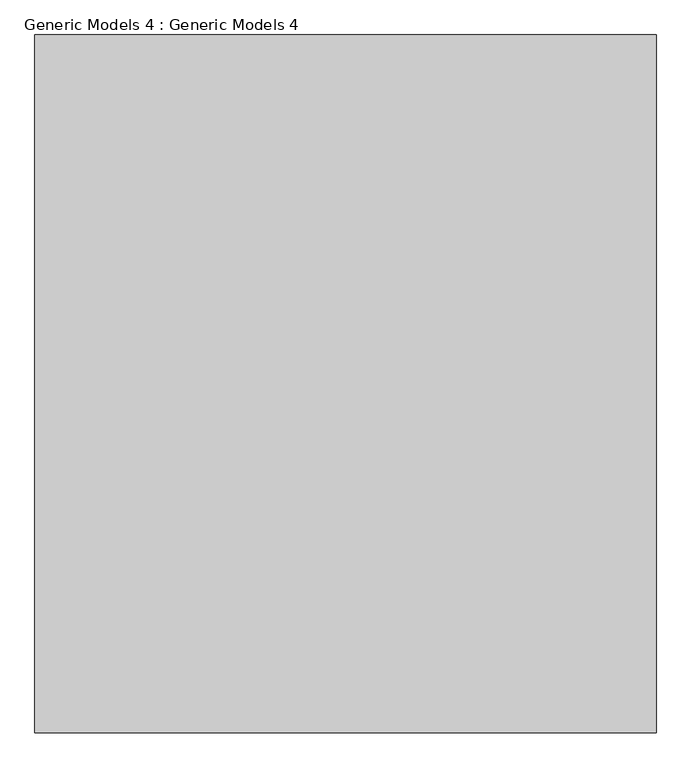
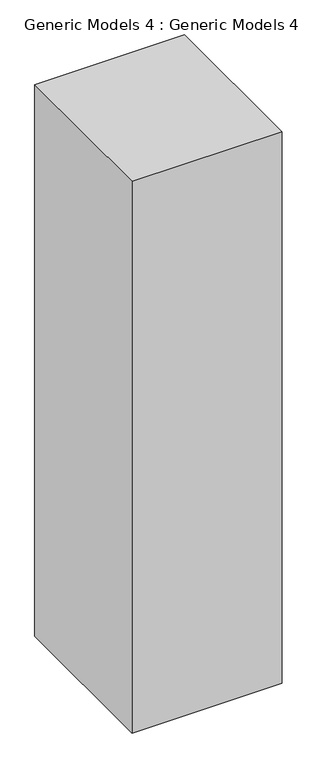
"""IFC4 building model written with IfcOpenShell, lengths in millimetres: proxy geometry, Generic Models 4 : Generic Models 4."""

from ifc_helpers import new_model, si_unit, frame, origin, place, context, project, spatial, polyline, outline, extrude, source, transform, mapped, element, save


def generic_models_4_generic_models_4_47707f26(model_context):
    return source(origin(), model_context, "Body", "SweptSolid", [
        extrude(outline(polyline([(-9125.6323769, -8681.0497532), (-9125.6323769, -9730.6391179), (-10060.7625896, -9730.6391179), (-10060.7625896, -8681.0497532), (-9125.6323769, -8681.0497532)])), frame((0.0, 0.0, 7450.2980542), z_axis=(0.0, 0.0, 1.0), x_axis=(1.0, 0.0, 0.0)), (0.0, 0.0, 1.0), 3635.301264),
    ])


if __name__ == "__main__":
    model = new_model("IFC4")
    model_context = context("Model", 3, world=origin())
    ifc_project = project(units=[si_unit("LENGTHUNIT", "METRE", prefix="MILLI")], contexts=[model_context])
    site = spatial("IfcSite", under=ifc_project)
    building = spatial("IfcBuilding", under=site)
    placement = place(None, origin())
    generic_models_4_generic_models_4_shape = generic_models_4_generic_models_4_47707f26(model_context)
    element("IfcBuildingElementProxy", 1, Name="Generic Models 4 : Generic Models 4", ObjectType="Generic Models 4 : Generic Models 4", at=placement, inside=building, context=model_context, shape_type="MappedRepresentation", body=[
        mapped(generic_models_4_generic_models_4_shape, transform((0.0, 0.0, 0.0), x_axis=(1.0, 0.0, 0.0), y_axis=(0.0, 1.0, 0.0), z_axis=(0.0, 0.0, 1.0))),
    ])
    save(model, "model.ifc")
